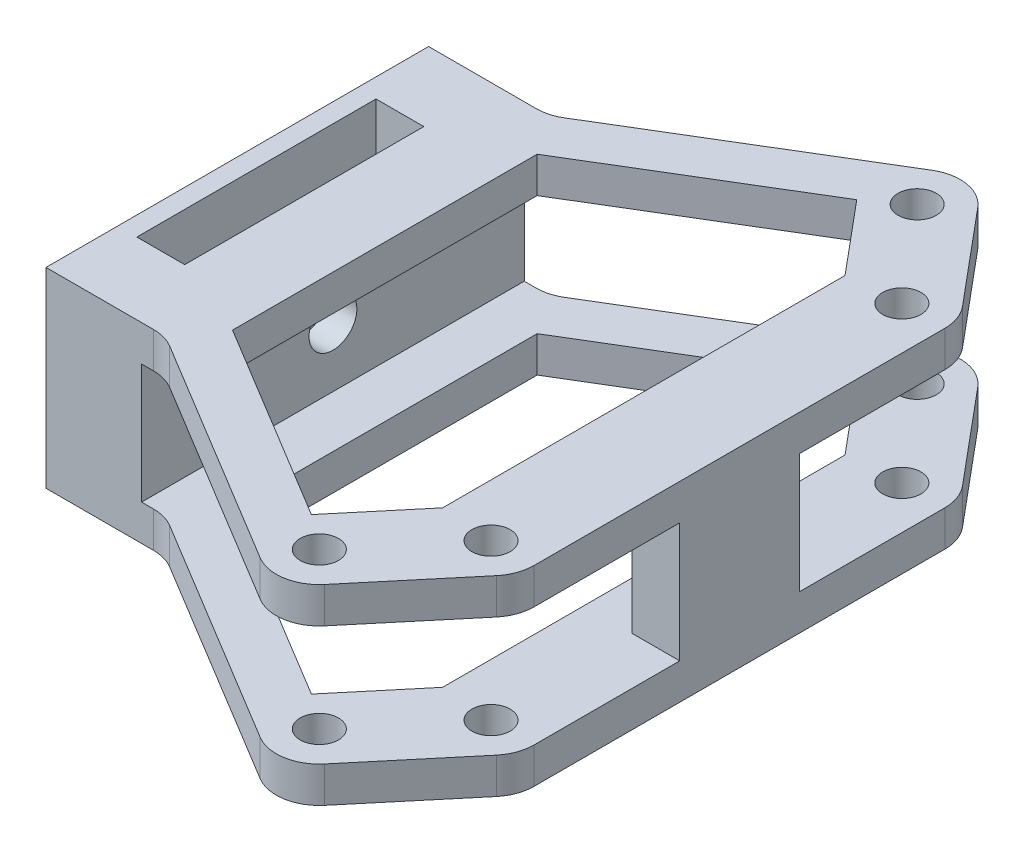
from build123d import *

# Parameters (mm, degrees)
FRAME_BODY_DEPTH                  = 20
WINDOW_AND_HOLES_SKETCH_R         = 4
WINDOW_AND_HOLES_SKETCH_W         = 10
WINDOW_AND_HOLES_SKETCH_H         = 50
WINDOW_AND_FIXING_HOLES_CUT_DEPTH = 20
SIDE_SLOT_SKETCH_W                = 75
SIDE_SLOT_SKETCH_H                = 25
SIDE_SLOT_CUT_DEPTH               = 100
TOP_SLOT_SKETCH_W                 = 59
TOP_SLOT_SKETCH_H                 = 25
TOP_SLOT_CUT_DEPTH                = 20
COUNTERBORE_24_SKETCH_R           = 12
COUNTERBORE_24_DEPTH              = 3
HOLE_10_SKETCH_R                  = 5
HOLE_10_DEPTH                     = 30
CORNER_FILLETS_R9_R               = 9


with BuildPart() as part:
    # Frame Profile Sketch → Frame Body (new, symmetric)
    with BuildSketch(Plane(origin=(0, 0, 0), x_dir=(1, 0, 0), z_dir=(0, 1, 0))):
        with BuildLine():
            Line((25, 40), (74.996258615, 70.203420742))
            ThreePointArc((74.996258615, 70.203420742), (81.13209258, 71.377128003), (86.553849817, 68.273807903))
            Line((86.553849817, 68.273807903), (102.903849817, 48.723807903))
            ThreePointArc((102.903849817, 48.723807903), (104.459747288, 46.02126616), (105, 42.95))
            Line((105, 42.95), (105, -42.95))
            ThreePointArc((105, -42.95), (104.459747288, -46.02126616), (102.903849817, -48.723807903))
            Line((102.903849817, -48.723807903), (86.553849817, -68.273807903))
            ThreePointArc((86.553849817, -68.273807903), (81.13209258, -71.377128003), (74.996258615, -70.203420742))
            Line((74.996258615, -70.203420742), (25, -40))
            Line((25, -40), (0, -40))
            Line((0, -40), (0, 40))
            Line((0, 40), (25, 40))
        make_face()
    extrude(amount=FRAME_BODY_DEPTH, both=True)

    # Window and Holes Sketch → Window and Fixing Holes Cut (cut, symmetric)
    with BuildSketch(Plane(origin=(0, 0, 0), x_dir=(1, 0, 0), z_dir=(0, 1, 0))):
        with Locations(Location((79.65, 62.5, 0), (0, 0, 270))):
            Circle(WINDOW_AND_HOLES_SKETCH_R)
        with Locations(Location((96, 42.95, 0), (0, 0, 270))):
            Circle(WINDOW_AND_HOLES_SKETCH_R)
        with Locations(Location((96, -42.95, 0), (0, 0, 270))):
            Circle(WINDOW_AND_HOLES_SKETCH_R)
        with Locations(Location((79.65, -62.5, 0), (0, 0, 270))):
            Circle(WINDOW_AND_HOLES_SKETCH_R)
        Polygon((30.85, 31.850943236), (30.85, -31.850943236), (72.504579862, -57.015042236), (85, -42.074035282), (85, 42.074035282), (72.504579862, 57.015042236), align=None)
        with Locations((9, 0)):
            Rectangle(WINDOW_AND_HOLES_SKETCH_W, WINDOW_AND_HOLES_SKETCH_H)
    extrude(amount=WINDOW_AND_FIXING_HOLES_CUT_DEPTH, both=True, mode=Mode.SUBTRACT)

    # Side Slot Sketch → Side Slot Cut (cut, symmetric)
    with BuildSketch(Plane.XY):
        with Locations((57.5, 0)):
            Rectangle(SIDE_SLOT_SKETCH_W, SIDE_SLOT_SKETCH_H)
    extrude(amount=SIDE_SLOT_CUT_DEPTH, both=True, mode=Mode.SUBTRACT)

    # Top Slot Sketch → Top Slot Cut (cut)
    with BuildSketch(Plane(origin=(105, 0, 0), x_dir=(0, 0, -1), z_dir=(1, 0, 0))):
        with Locations((-42, 0)):
            Rectangle(TOP_SLOT_SKETCH_W, TOP_SLOT_SKETCH_H)
        with Locations((42, 0)):
            Rectangle(TOP_SLOT_SKETCH_W, TOP_SLOT_SKETCH_H)
    extrude(amount=-TOP_SLOT_CUT_DEPTH, mode=Mode.SUBTRACT)

    # Counterbore Ø24 Sketch → Counterbore Ø24 (cut)
    with BuildSketch(Plane.ZY):
        Circle(COUNTERBORE_24_SKETCH_R)
    extrude(amount=-COUNTERBORE_24_DEPTH, mode=Mode.SUBTRACT)

    # Hole Ø10 Sketch → Hole Ø10 (cut)
    with BuildSketch(Plane.ZY.offset(-3)):
        with Locations(Location((0, 0, 0), (0, 0, 270))):
            Circle(HOLE_10_SKETCH_R)
    extrude(amount=-HOLE_10_DEPTH, mode=Mode.SUBTRACT)

    # Corner Fillets R9
    corner_fillets_r9_edges = [part.edges().sort_by_distance(p)[0] for p in [
        (25, -16.25, -40),
        (25, -16.25, 40),
        (25, 16.25, -40),
        (25, 16.25, 40),
    ]]
    fillet(corner_fillets_r9_edges, radius=CORNER_FILLETS_R9_R)


solid = part.part
